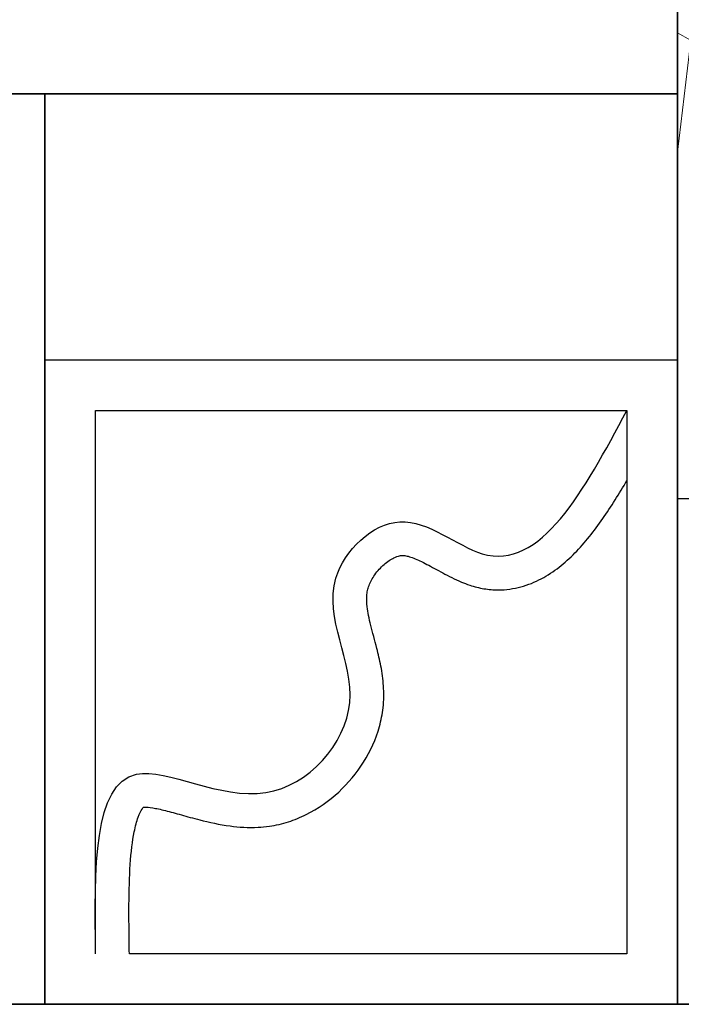
# Model space of a CAD drawing. Units: inches. Extents: x 3 to 303, y 4 to 326.
# Tile 2 of 6: x 141 to 220, y 4 to 120. Entities that reach past the tile are written whole.
import ezdxf

# ---------------------------------------------------------------- set-up
doc = ezdxf.new("R2010")
doc.units = ezdxf.units.IN
doc.header["$MEASUREMENT"] = 0
for name, color, linetype, lineweight in [('A-DOOR', 3, 'Continuous', 25), ('A-ELEV', 7, 'Continuous', 35), ('A-ELEV-FENC', 8, 'Continuous', 25), ('A-ELEV-PATT', 8, 'Continuous', 13)]:
    doc.layers.add(name, color=color, linetype=linetype, lineweight=lineweight)

msp = doc.modelspace()

# ---------------------------------------------------------------- hatches: boundary and pattern name
at = {"layer": 'A-ELEV-PATT'}
h = msp.add_hatch(dxfattribs=at)
h.set_pattern_fill('GRAVEL', color=256, scale=150, angle=90)
h.set_pattern_definition([(318.0128, (-159.712, 82.498), (1350, -1200), [20.18, -1997.863]), (274.9697, (-144.712, 68.998), (-150, 1800), [34.63, -3428.3887]), (222.5104, (-141.712, 34.498), (1650, 1500), [24.418, -2417.405]), (357.2737, (-104.212, -24.002), (-3000, 150), [31.536, -3122.034]), (22.8337, (-72.712, -25.502), (-1800, -750), [30.923, -3061.406]), (87.2737, (-44.212, -13.502), (-150, -3000), [31.536, -3122.034]), (127.6942, (-42.712, 17.9977), (1500, -1950), [41.7043, -4128.7273]), (162.2553, (-68.212, 50.998), (-3300, 1050), [39.373, -3897.948]), (211.4296, (-105.712, 62.998), (-1950, -1200), [31.6425, -3132.611]), (265.2364, (-132.712, 46.498), (150, 1650), [36.125, -1770.114]), (312.3974, (-135.712, 10.4977), (1650, -1800), [46.717, -4625.0063]), (228.814, (-102.712, 124.498), (-900, -1050), [15.945, -1578.577]), (261.4692, (-113.212, 112.498), (300, 1950), [30.3356, -3003.227]), (315, (-117.71, 82.5), (150, -3e-14), [21.213, -190.92]), (293.1986, (-135.712, 71.998), (-300, 750), [11.424, -1130.942]), (21.8014, (-131.212, 61.498), (-450, -150), [16.155, -791.62]), (120.964, (-116.212, 67.498), (-300, 450), [26.24, -848.403]), (251.565, (-129.71, 90), (150, 300), [18.974, -455.368]), (106.3895, (-131.212, -25.502), (-450, 1500), [26.58, -2631.427]), (160.3462, (-138.712, -0.002), (1650, -600), [22.299, -2207.611]), (23.1986, (-159.712, 89.998), (-750, -300), [22.847, -1119.519]), (73.6105, (-138.712, 98.998), (-450, -1500), [26.58, -2631.427]), (69.444, (-38.212, -25.502), (-300, -750), [25.632, -1255.969]), (24.7751, (-29.212, -1.502), (-1650, -750), [21.477, -2126.1965]), (156.8014, (-9.712, 91.498), (-750, 300), [22.847, -1119.519]), (107.354, (-30.712, 100.498), (600, -1950), [25.145, -2489.3135]), (159.444, (-9.712, 17.998), (750, -300), [12.816, -1268.785]), (191.31, (-9.712, 82.498), (-600, -150), [7.649, -757.204]), (255.964, (-17.21, 80.998), (150, 450), [30.923, -587.543]), (276.009, (-24.712, 50.998), (-150, 1500), [28.6575, -2837.0885]), (33.69, (-102.71, 67.498), (-300, -150), [21.633, -519.2]), (83.1572, (-84.712, 79.498), (300, 2550), [37.769, -3739.1344]), (150.9454, (-80.212, 116.998), (1050, -600), [15.443, -1528.901]), (180, (-93.71, 124.5), (-150, -150), [9, -141]), (210.2564, (-29.212, 47.998), (1050, 600), [20.839, -2063.028]), (138.0128, (-47.212, 37.498), (-1350, 1200), [40.361, -1977.683]), (90, (-77.21, 64.5), (-150, 150), [39, -111]), (55.3048, (-77.212, 103.498), (1050, 1500), [23.717, -2347.991]), (344.0546, (-63.712, 122.998), (600, -150), [21.84, -1070.176]), (297.646, (-42.712, 116.998), (1500, -2850), [35.56, -3520.421]), (265.426, (-26.212, 85.498), (-150, -1950), [37.62, -3724.361])])
h.paths.add_polyline_path([(303.23, 123.62), (303.23, 243.62), (303.23, 325.61), (219.23, 325.61), (219.23, 243.62), (219.23, 63.62), (232.73, 63.62), (232.73, 80.06), (244.07, 80.06), (244.07, 63.62), (257.57, 63.62), (257.57, 80.06), (268.91, 80.06), (268.91, 63.62), (282.42, 63.62), (282.42, 80.06), (293.76, 80.06), (293.76, 63.62), (303.23, 63.62)])
h.paths.add_polyline_path([(286.72, 105.38), (238.22, 105.38), (238.22, 300.66), (286.72, 300.66)], flags=16)
h.paths.add_polyline_path([(280.72, 111.38), (244.22, 111.38), (244.22, 294.66), (280.72, 294.66)], flags=0)

# ---------------------------------------------------------------- linework, layer by layer
at = {"layer": 'A-DOOR'}
msp.add_lwpolyline([(144.23, 80.06), (219.23, 80.06), (219.23, 3.62), (144.23, 3.62)], close=True, dxfattribs=at)
for points in [[(150.23, 9.62), (150.23, 74.06), (213.23, 74.06)], [(213.23, 74.06), (213.23, 9.62), (154.23, 9.62)]]:
    msp.add_lwpolyline(points, dxfattribs=at)
for points, knots in [([(150.23, 9.62), (150.09, 19.72), (149.86, 37), (170.89, 24.29), (184.34, 39.52), (174.84, 52.71), (186.47, 64), (200.8, 50.86), (208.12, 64.52), (213.23, 74.06)], [0, 0, 0, 0, 21.819862, 37.325187, 51.887363, 66.774149, 76.880374, 87.344603, 111.497762, 111.497762, 111.497762, 111.497762]), ([(155.91, 26.98), (155.94, 26.99), (155.99, 26.99), (156.26, 27), (156.58, 26.98), (157.42, 26.85), (157.93, 26.74), (159.08, 26.45), (159.71, 26.27), (161.08, 25.89), (161.81, 25.69), (163.7, 25.21), (164.9, 24.94), (167.23, 24.63), (168.34, 24.56), (169.93, 24.64), (170.38, 24.68), (171.22, 24.8), (171.6, 24.87), (172.36, 25.05), (172.73, 25.15), (173.82, 25.5), (174.52, 25.79), (176.62, 26.83), (177.91, 27.74), (180.19, 29.85), (181.18, 31.04), (182.82, 33.66), (183.47, 35.07), (184.08, 37.29), (184.23, 38.03), (184.37, 39.23), (184.39, 39.67), (184.41, 40.54), (184.39, 40.96), (184.31, 42.19), (184.2, 42.97), (183.92, 44.46), (183.75, 45.16), (183.33, 46.81), (183.07, 47.72), (182.66, 49.37), (182.51, 50.12), (182.38, 51.25), (182.36, 51.67), (182.4, 52.28), (182.43, 52.5), (182.52, 52.9), (182.57, 53.08), (182.8, 53.68), (183.04, 54.13), (183.66, 55.01), (184.03, 55.43), (184.82, 56.12), (185.23, 56.4), (185.85, 56.7), (186.09, 56.78), (186.35, 56.84), (186.42, 56.85), (186.53, 56.86), (186.57, 56.86), (186.68, 56.86), (186.74, 56.85), (186.94, 56.83), (187.1, 56.8), (187.49, 56.7), (187.71, 56.63), (188.41, 56.36), (188.94, 56.1), (190.09, 55.5), (190.72, 55.14), (192.07, 54.42), (192.8, 54.04), (193.92, 53.57), (194.25, 53.44), (194.87, 53.24), (195.15, 53.16), (195.71, 53.02), (195.99, 52.96), (196.84, 52.82), (197.4, 52.77), (198.89, 52.77), (199.8, 52.9), (201.51, 53.36), (202.32, 53.69), (203.83, 54.49), (204.53, 54.96), (205.85, 55.99), (206.47, 56.55), (208.26, 58.37), (209.34, 59.75), (211.36, 62.65), (212.31, 64.18), (213.23, 65.76)], [22.186302, 22.186302, 22.186302, 22.186302, 23.035301, 23.035301, 25.021695, 25.021695, 27.008088, 27.008088, 28.994482, 28.994482, 30.980875, 30.980875, 33.875903, 33.875903, 36.261668, 36.261668, 37.174934, 37.174934, 37.95302, 37.95302, 38.731105, 38.731105, 40.287275, 40.287275, 43.580394, 43.580394, 46.873512, 46.873512, 50.166631, 50.166631, 51.746175, 51.746175, 52.675627, 52.675627, 53.605079, 53.605079, 55.463983, 55.463983, 57.322887, 57.322887, 60.075665, 60.075665, 62.828443, 62.828443, 64.869314, 64.869314, 66.143342, 66.143342, 67.304795, 67.304795, 69.633921, 69.633921, 71.963046, 71.963046, 74.292171, 74.292171, 75.985188, 75.985188, 76.667214, 76.667214, 77.236276, 77.236276, 77.805338, 77.805338, 78.943462, 78.943462, 80.081586, 80.081586, 82.149442, 82.149442, 84.217297, 84.217297, 86.285152, 86.285152, 87.093976, 87.093976, 87.720891, 87.720891, 88.347806, 88.347806, 89.601636, 89.601636, 91.651231, 91.651231, 93.700826, 93.700826, 95.750421, 95.750421, 97.800016, 97.800016, 101.985659, 101.985659, 106.077072, 106.077072, 106.077072, 106.077072]), ([(154.23, 9.62), (154.23, 9.63), (154.23, 9.65), (154.23, 9.66), (154.23, 9.66), (154.23, 9.67), (154.23, 9.67), (154.22, 10.32), (154.21, 10.97), (154.19, 12.91), (154.18, 14.18), (154.2, 17.11), (154.24, 18.73), (154.44, 21.67), (154.6, 22.99), (154.95, 24.75), (155.11, 25.34), (155.44, 26.25), (155.61, 26.57), (155.82, 26.89), (155.88, 26.96), (155.91, 26.98)], [-0.038741, -0.038741, -0.038741, -0.038741, -0.008495, -0.008495, -0.008495, 0, 0, 0, 1.410757, 1.410757, 4.232272, 4.232272, 8.152598, 8.152598, 12.072924, 12.072924, 14.555292, 14.555292, 17.03766, 17.03766, 18.725413, 18.725413, 18.725413, 18.725413])]:
    msp.add_open_spline(points, degree=3, knots=knots, dxfattribs=at)
at = {"layer": 'A-ELEV'}
for p, q in [((219.23, 3.62), (219.23, 243.62)), ((15.23, 111.62), (219.23, 111.62)), ((144.23, 3.62), (144.23, 111.62)), ((15.23, 3.62), (303.23, 3.62))]:
    msp.add_line(p, q, dxfattribs=at)
at = {"layer": 'A-ELEV-FENC'}
msp.add_lwpolyline([(293.76, 63.62), (303.23, 63.62), (303.23, 3.62), (219.23, 3.62), (219.23, 63.62), (232.73, 63.62)], dxfattribs=at)

doc.saveas('drawing.dxf')
